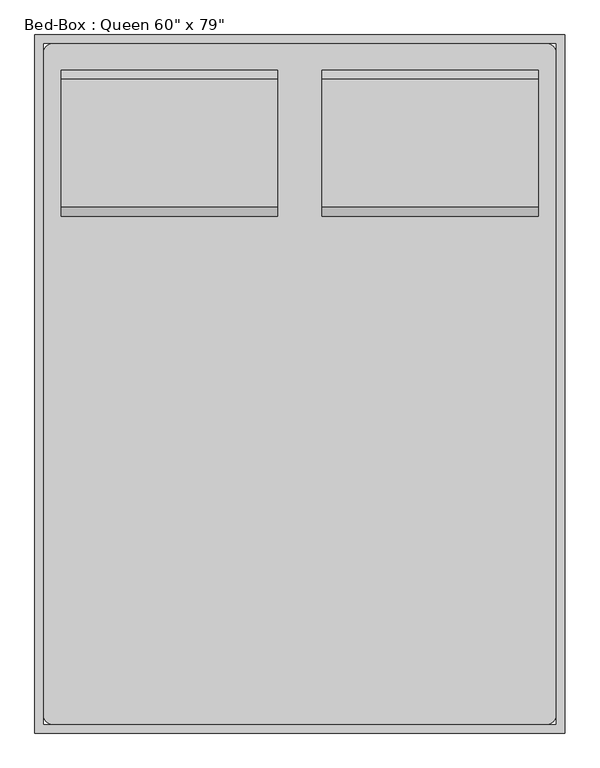
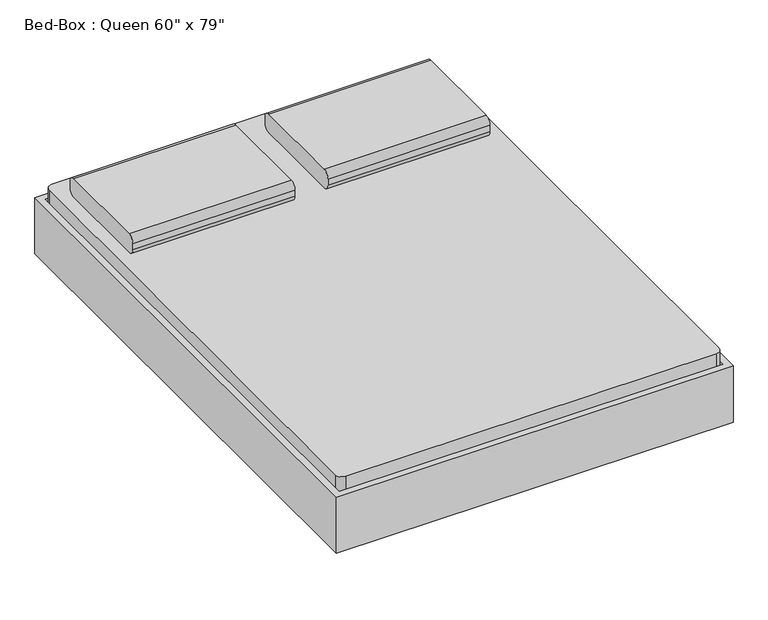
"""IFC4 building model written with IfcOpenShell, lengths in millimetres: furniture geometry."""

from ifc_helpers import new_model, si_unit, point, frame, frame_2d, origin, place, context, project, spatial, polyline, circle_curve, trimmed, segment, composite_curve, outline, extrude, source, transform, mapped, element, save
from ifc_brep_helpers import plane_surface, cylinder_surface, revolved_surface, advanced_brep


def furniture_1d2926bd(model_context):
    return source(origin(), model_context, "Body", "SolidModel", [
        extrude(outline(composite_curve([segment(polyline([(641.8704918, 406.4), (273.5704918, 406.4)]), True, "CONTINUOUS"), segment(trimmed(circle_curve(frame_2d((273.5704918, 431.8)), 25.4), [point((273.5704918, 406.4))], [point((248.1704918, 431.8))], False, "CARTESIAN"), True, "CONTINUOUS"), segment(polyline([(248.1704918, 431.8), (248.1704918, 457.2)]), True, "CONTINUOUS"), segment(trimmed(circle_curve(frame_2d((273.5704918, 457.2)), 25.4), [point((248.1704918, 457.2))], [point((273.5704918, 482.6))], False, "CARTESIAN"), True, "CONTINUOUS"), segment(polyline([(273.5704918, 482.6), (641.8704918, 482.6)]), True, "CONTINUOUS"), segment(trimmed(circle_curve(frame_2d((641.8704918, 457.2)), 25.4), [point((641.8704918, 482.6))], [point((667.2704918, 457.2))], False, "CARTESIAN"), True, "CONTINUOUS"), segment(polyline([(667.2704918, 457.2), (667.2704918, 431.8)]), True, "CONTINUOUS"), segment(trimmed(circle_curve(frame_2d((641.8704918, 431.8)), 25.4), [point((667.2704918, 431.8))], [point((641.8704918, 406.4))], False, "CARTESIAN"), True, "CONTINUOUS")], self_intersect=False)), frame((402.652459, 0.0, 0.0), z_axis=(1.0, 0.0, 0.0), x_axis=(0.0, 1.0, 0.0)), (0.0, 0.0, 1.0), 622.3),
        extrude(outline(composite_curve([segment(polyline([(641.8704918, 406.4), (273.5704918, 406.4)]), True, "CONTINUOUS"), segment(trimmed(circle_curve(frame_2d((273.5704918, 431.8)), 25.4), [point((273.5704918, 406.4))], [point((248.1704918, 431.8))], False, "CARTESIAN"), True, "CONTINUOUS"), segment(polyline([(248.1704918, 431.8), (248.1704918, 457.2)]), True, "CONTINUOUS"), segment(trimmed(circle_curve(frame_2d((273.5704918, 457.2)), 25.4), [point((248.1704918, 457.2))], [point((273.5704918, 482.6))], False, "CARTESIAN"), True, "CONTINUOUS"), segment(polyline([(273.5704918, 482.6), (641.8704918, 482.6)]), True, "CONTINUOUS"), segment(trimmed(circle_curve(frame_2d((641.8704918, 457.2)), 25.4), [point((641.8704918, 482.6))], [point((667.2704918, 457.2))], False, "CARTESIAN"), True, "CONTINUOUS"), segment(polyline([(667.2704918, 457.2), (667.2704918, 431.8)]), True, "CONTINUOUS"), segment(trimmed(circle_curve(frame_2d((641.8704918, 431.8)), 25.4), [point((667.2704918, 431.8))], [point((641.8704918, 406.4))], False, "CARTESIAN"), True, "CONTINUOUS")], self_intersect=False)), frame((-346.647541, 0.0, 0.0), z_axis=(1.0, 0.0, 0.0), x_axis=(0.0, 1.0, 0.0)), (0.0, 0.0, 1.0), 622.3),
        advanced_brep(
        [(-397.1231784, 514.8704918, 177.8), (-397.1231784, 438.6704918, 177.8), (-397.1231784, 438.6704918, 196.85), (-397.1231784, 514.8704918, 196.85), (-346.3231784, 514.8704918, 177.8), (-346.3231784, 438.6704918, 177.8), (-334.1869899, 438.6704918, 196.85), (-334.1869899, 514.8704918, 196.85), (-270.2523099, 514.8704918, 14.6654962), (-270.2523099, 438.6704918, 14.6654962), (-252.9871466, 438.6704918, 22.716374), (-252.9871466, 514.8704918, 22.716374), (-247.2320921, 438.6704918, 0.0), (-247.2320921, 514.8704918, 0.0), (-247.2320921, 438.6704918, 19.05), (-247.2320921, 514.8704918, 19.05), (-168.6195862, 514.8704918, 0.0), (-168.6195862, 438.6704918, 0.0), (-168.6195862, 438.6704918, 19.05), (-168.6195862, 514.8704918, 19.05), (-155.9195862, 438.6704918, 3.4029547), (-155.9195862, 514.8704918, 3.4029547), (-165.4445862, 438.6704918, 19.9007387), (-165.4445862, 514.8704918, 19.9007387), (-95.822541, 514.8704918, 38.1), (-95.822541, 438.6704918, 38.1), (-100.9269731, 438.6704918, 57.15), (-100.9269731, 514.8704918, 57.15), (774.4518216, 514.8704918, 38.1), (774.4518216, 438.6704918, 38.1), (779.5562537, 438.6704918, 57.15), (779.5562537, 514.8704918, 57.15), (834.5488669, 514.8704918, 3.4029547), (834.5488669, 438.6704918, 3.4029547), (844.0738669, 438.6704918, 19.9007387), (844.0738669, 514.8704918, 19.9007387), (847.2488669, 438.6704918, 0.0), (847.2488669, 514.8704918, 0.0), (847.2488669, 438.6704918, 19.05), (847.2488669, 514.8704918, 19.05), (925.8613728, 514.8704918, 0.0), (925.8613728, 438.6704918, 0.0), (925.8613728, 438.6704918, 19.05), (925.8613728, 514.8704918, 19.05), (948.8815906, 438.6704918, 14.6654962), (948.8815906, 514.8704918, 14.6654962), (931.6164272, 438.6704918, 22.716374), (931.6164272, 514.8704918, 22.716374), (1024.952459, 514.8704918, 177.8), (1024.952459, 438.6704918, 177.8), (1012.8162705, 438.6704918, 196.85), (1012.8162705, 514.8704918, 196.85), (1075.752459, 514.8704918, 177.8), (1075.752459, 514.8704918, 196.85), (1075.752459, 438.6704918, 196.85), (1075.752459, 438.6704918, 177.8)],
        [
            (0, 1),
            (1, 2),
            (2, 3),
            (3, 0),
            (0, 4),
            (4, 5),
            (5, 1),
            (5, 6),
            (6, 2),
            (6, 7),
            (7, 3),
            (7, 4),
            (4, 8),
            (8, 9),
            (9, 5),
            (9, 10),
            (10, 6),
            (10, 11),
            (11, 7),
            (11, 8),
            (12, 9, circle_curve(frame((-247.2320921, 438.6704918, 25.4), z_axis=(0.0, 1.0, 0.0), x_axis=(-0.9063077870366486, 0.0, -0.42261826174070233)), 25.4)),
            (8, 13, circle_curve(frame((-247.2320921, 514.8704918, 25.4), z_axis=(0.0, -1.0, 0.0), x_axis=(-0.9063077870366486, 0.0, -0.42261826174070233)), 25.4)),
            (13, 12),
            (14, 10, circle_curve(frame((-247.2320921, 438.6704918, 25.4), z_axis=(0.0, 1.0, 0.0), x_axis=(-0.9063077870366486, 0.0, -0.42261826174070233)), 6.35)),
            (12, 14),
            (15, 11, circle_curve(frame((-247.2320921, 514.8704918, 25.4), z_axis=(0.0, 1.0, 0.0), x_axis=(-0.9063077870366486, 0.0, -0.42261826174070233)), 6.35)),
            (14, 15),
            (15, 13),
            (13, 16),
            (16, 17),
            (17, 12),
            (17, 18),
            (18, 14),
            (18, 19),
            (19, 15),
            (19, 16),
            (20, 17, circle_curve(frame((-168.6195862, 438.6704918, 25.4), z_axis=(0.0, 1.0, 0.0), x_axis=(0.0, 0.0, -1.0)), 25.4)),
            (16, 21, circle_curve(frame((-168.6195862, 514.8704918, 25.4), z_axis=(0.0, -1.0, 0.0), x_axis=(0.0, 0.0, -1.0)), 25.4)),
            (21, 20),
            (22, 18, circle_curve(frame((-168.6195862, 438.6704918, 25.4), z_axis=(0.0, 1.0, 0.0), x_axis=(0.0, 0.0, -1.0)), 6.35)),
            (20, 22),
            (23, 19, circle_curve(frame((-168.6195862, 514.8704918, 25.4), z_axis=(0.0, 1.0, 0.0), x_axis=(0.0, 0.0, -1.0)), 6.35)),
            (22, 23),
            (23, 21),
            (21, 24),
            (24, 25),
            (25, 20),
            (25, 26),
            (26, 22),
            (26, 27),
            (27, 23),
            (27, 24),
            (24, 28),
            (28, 29),
            (29, 25),
            (29, 30),
            (30, 26),
            (30, 31),
            (31, 27),
            (31, 28),
            (28, 32),
            (32, 33),
            (33, 29),
            (33, 34),
            (34, 30),
            (34, 35),
            (35, 31),
            (35, 32),
            (36, 33, circle_curve(frame((847.2488669, 438.6704918, 25.4), z_axis=(0.0, 1.0, 0.0), x_axis=(-0.5000000000000463, 0.0, -0.8660254037844118)), 25.4)),
            (32, 37, circle_curve(frame((847.2488669, 514.8704918, 25.4), z_axis=(0.0, -1.0, 0.0), x_axis=(-0.5000000000000463, 0.0, -0.8660254037844118)), 25.4)),
            (37, 36),
            (38, 34, circle_curve(frame((847.2488669, 438.6704918, 25.4), z_axis=(0.0, 1.0, 0.0), x_axis=(-0.5000000000000463, 0.0, -0.8660254037844118)), 6.35)),
            (36, 38),
            (39, 35, circle_curve(frame((847.2488669, 514.8704918, 25.4), z_axis=(0.0, 1.0, 0.0), x_axis=(-0.5000000000000463, 0.0, -0.8660254037844118)), 6.35)),
            (38, 39),
            (39, 37),
            (37, 40),
            (40, 41),
            (41, 36),
            (41, 42),
            (42, 38),
            (42, 43),
            (43, 39),
            (43, 40),
            (44, 41, circle_curve(frame((925.8613728, 438.6704918, 25.4), z_axis=(0.0, 1.0, 0.0), x_axis=(0.0, 0.0, -1.0)), 25.4)),
            (40, 45, circle_curve(frame((925.8613728, 514.8704918, 25.4), z_axis=(0.0, -1.0, 0.0), x_axis=(0.0, 0.0, -1.0)), 25.4)),
            (45, 44),
            (46, 42, circle_curve(frame((925.8613728, 438.6704918, 25.4), z_axis=(0.0, 1.0, 0.0), x_axis=(0.0, 0.0, -1.0)), 6.35)),
            (44, 46),
            (47, 43, circle_curve(frame((925.8613728, 514.8704918, 25.4), z_axis=(0.0, 1.0, 0.0), x_axis=(0.0, 0.0, -1.0)), 6.35)),
            (46, 47),
            (47, 45),
            (45, 48),
            (48, 49),
            (49, 44),
            (49, 50),
            (50, 46),
            (50, 51),
            (51, 47),
            (51, 48),
            (52, 53),
            (53, 54),
            (54, 55),
            (55, 52),
            (48, 52),
            (55, 49),
            (54, 50),
            (53, 51),
        ],
        [
            plane_surface(frame((-397.1231784, 768.8704918, -152.9490627), z_axis=(-1.0, 0.0, 0.0), x_axis=(0.0, 1.0, 0.0))),
            plane_surface(frame((-397.1231784, 514.8704918, 177.8), z_axis=(0.0, 0.0, -1.0), x_axis=(1.0, 0.0, 0.0))),
            plane_surface(frame((-397.1231784, 438.6704918, 177.8), z_axis=(0.0, -1.0, 0.0), x_axis=(1.0, 0.0, 0.0))),
            plane_surface(frame((-397.1231784, 438.6704918, 196.85), z_axis=(0.0, 0.0, 1.0), x_axis=(1.0, 0.0, 0.0))),
            plane_surface(frame((-397.1231784, 514.8704918, 196.85), z_axis=(0.0, 1.0, 0.0), x_axis=(1.0, 0.0, 0.0))),
            plane_surface(frame((-346.3231784, 514.8704918, 177.8), z_axis=(-0.9063077870366485, 0.0, -0.4226182617407027), x_axis=(0.4226182617407027, 0.0, -0.9063077870366485))),
            plane_surface(frame((-346.3231784, 438.6704918, 177.8), z_axis=(0.0, -1.0, 0.0), x_axis=(0.4226182617407025, 0.0, -0.9063077870366486))),
            plane_surface(frame((-334.1869899, 438.6704918, 196.85), z_axis=(0.9063077870366484, 0.0, 0.4226182617407028), x_axis=(0.4226182617407028, 0.0, -0.9063077870366484))),
            plane_surface(frame((-334.1869899, 514.8704918, 196.85), z_axis=(0.0, 1.0, 0.0), x_axis=(0.42261826174070277, 0.0, -0.9063077870366485))),
            cylinder_surface(frame((-247.2320921, 768.8704918, 25.4), z_axis=(0.0, -1.0, 0.0), x_axis=(-0.9063077870366486, 0.0, -0.42261826174070233)), 25.4),
            plane_surface(frame((-247.2320921, 438.6704918, 25.4), z_axis=(0.0, -1.0, 0.0), x_axis=(-0.9063077870366486, 0.0, -0.42261826174070233))),
            revolved_surface(polyline([(-252.9871465476827, 438.6704918, 22.71637403794654), (-252.9871465476827, 514.8704918, 22.71637403794654)]), (-247.2320921, 768.8704918, 25.4), (0.0, -1.0, 0.0)),
            plane_surface(frame((-247.2320921, 514.8704918, 25.4), z_axis=(0.0, 1.0, 0.0), x_axis=(-0.9063077870366486, 0.0, -0.42261826174070233))),
            plane_surface(frame((-247.2320921, 514.8704918, 0.0), z_axis=(0.0, 0.0, -1.0), x_axis=(1.0, 0.0, 0.0))),
            plane_surface(frame((-247.2320921, 438.6704918, 0.0), z_axis=(0.0, -1.0, 0.0), x_axis=(1.0, 0.0, 0.0))),
            plane_surface(frame((-247.2320921, 438.6704918, 19.05), z_axis=(0.0, 0.0, 1.0), x_axis=(1.0, 0.0, 0.0))),
            plane_surface(frame((-247.2320921, 514.8704918, 19.05), z_axis=(0.0, 1.0, 0.0), x_axis=(1.0, 0.0, 0.0))),
            cylinder_surface(frame((-168.6195862, 768.8704918, 25.4), z_axis=(0.0, -1.0, 0.0), x_axis=(0.0, 0.0, -1.0)), 25.4),
            plane_surface(frame((-168.6195862, 438.6704918, 25.4), z_axis=(0.0, -1.0, 0.0), x_axis=(0.0, 0.0, -1.0))),
            revolved_surface(polyline([(-168.6195862, 438.6704918, 19.049999999999997), (-168.6195862, 514.8704918, 19.049999999999997)]), (-168.6195862, 768.8704918, 25.4), (0.0, -1.0, 0.0)),
            plane_surface(frame((-168.6195862, 514.8704918, 25.4), z_axis=(0.0, 1.0, 0.0), x_axis=(0.0, 0.0, -1.0))),
            plane_surface(frame((-155.9195862, 514.8704918, 3.4029547), z_axis=(0.49999999999988004, 0.0, -0.866025403784508), x_axis=(0.866025403784508, 0.0, 0.49999999999988004))),
            plane_surface(frame((-155.9195862, 438.6704918, 3.4029547), z_axis=(0.0, -1.0, 0.0), x_axis=(0.8660254037845078, 0.0, 0.49999999999988026))),
            plane_surface(frame((-165.4445862, 438.6704918, 19.9007387), z_axis=(-0.4999999999998799, 0.0, 0.866025403784508), x_axis=(0.866025403784508, 0.0, 0.4999999999998799))),
            plane_surface(frame((-165.4445862, 514.8704918, 19.9007387), z_axis=(0.0, 1.0, 0.0), x_axis=(0.8660254037845075, 0.0, 0.49999999999988076))),
            plane_surface(frame((-95.822541, 514.8704918, 38.1), z_axis=(0.0, 0.0, -1.0), x_axis=(1.0, 0.0, 0.0))),
            plane_surface(frame((-95.822541, 438.6704918, 38.1), z_axis=(0.0, -1.0, 0.0), x_axis=(1.0, 0.0, 0.0))),
            plane_surface(frame((-100.9269731, 438.6704918, 57.15), z_axis=(0.0, 0.0, 1.0), x_axis=(1.0, 0.0, 0.0))),
            plane_surface(frame((-100.9269731, 514.8704918, 57.15), z_axis=(0.0, 1.0, 0.0), x_axis=(1.0, 0.0, 0.0))),
            plane_surface(frame((774.4518216, 514.8704918, 38.1), z_axis=(-0.5000000000000455, 0.0, -0.8660254037844125), x_axis=(0.8660254037844125, 0.0, -0.5000000000000455))),
            plane_surface(frame((774.4518216, 438.6704918, 38.1), z_axis=(0.0, -1.0, 0.0), x_axis=(0.866025403784412, 0.0, -0.5000000000000463))),
            plane_surface(frame((779.5562537, 438.6704918, 57.15), z_axis=(0.5000000000000466, 0.0, 0.8660254037844117), x_axis=(0.8660254037844117, 0.0, -0.5000000000000466))),
            plane_surface(frame((779.5562537, 514.8704918, 57.15), z_axis=(0.0, 1.0, 0.0), x_axis=(0.8660254037844115, 0.0, -0.5000000000000471))),
            cylinder_surface(frame((847.2488669, 768.8704918, 25.4), z_axis=(0.0, -1.0, 0.0), x_axis=(-0.5000000000000463, 0.0, -0.8660254037844118)), 25.4),
            plane_surface(frame((847.2488669, 438.6704918, 25.4), z_axis=(0.0, -1.0000000000000002, 0.0), x_axis=(-0.5000000000000464, 0.0, -0.866025403784412))),
            revolved_surface(polyline([(844.0738668999998, 438.6704918, 19.90073868596898), (844.0738668999998, 514.8704918, 19.90073868596898)]), (847.2488669, 768.8704918, 25.4), (0.0, -1.0, 0.0)),
            plane_surface(frame((847.2488669, 514.8704918, 25.4), z_axis=(0.0, 1.0000000000000002, 0.0), x_axis=(-0.5000000000000464, 0.0, -0.866025403784412))),
            plane_surface(frame((847.2488669, 514.8704918, 0.0), z_axis=(0.0, 0.0, -1.0), x_axis=(1.0, 0.0, 0.0))),
            plane_surface(frame((847.2488669, 438.6704918, 0.0), z_axis=(0.0, -1.0, 0.0), x_axis=(1.0, 0.0, 0.0))),
            plane_surface(frame((847.2488669, 438.6704918, 19.05), z_axis=(0.0, 0.0, 1.0), x_axis=(1.0, 0.0, 0.0))),
            plane_surface(frame((847.2488669, 514.8704918, 19.05), z_axis=(0.0, 1.0, 0.0), x_axis=(1.0, 0.0, 0.0))),
            cylinder_surface(frame((925.8613728, 768.8704918, 25.4), z_axis=(0.0, -1.0, 0.0), x_axis=(0.0, 0.0, -1.0)), 25.4),
            plane_surface(frame((925.8613728, 438.6704918, 25.4), z_axis=(0.0, -1.0, 0.0), x_axis=(0.0, 0.0, -1.0))),
            revolved_surface(polyline([(925.8613728, 438.6704918, 19.049999999999997), (925.8613728, 514.8704918, 19.049999999999997)]), (925.8613728, 768.8704918, 25.4), (0.0, -1.0, 0.0)),
            plane_surface(frame((925.8613728, 514.8704918, 25.4), z_axis=(0.0, 1.0, 0.0), x_axis=(0.0, 0.0, -1.0))),
            plane_surface(frame((948.8815906, 514.8704918, 14.6654962), z_axis=(0.90630778703668, 0.0, -0.42261826174063505), x_axis=(0.42261826174063505, 0.0, 0.90630778703668))),
            plane_surface(frame((948.8815906, 438.6704918, 14.6654962), z_axis=(0.0, -1.0, 0.0), x_axis=(0.42261826174063566, 0.0, 0.9063077870366797))),
            plane_surface(frame((931.6164272, 438.6704918, 22.716374), z_axis=(-0.9063077870366801, 0.0, 0.42261826174063477), x_axis=(0.42261826174063477, 0.0, 0.9063077870366801))),
            plane_surface(frame((931.6164272, 514.8704918, 22.716374), z_axis=(0.0, 1.0, 0.0), x_axis=(0.4226182617406345, 0.0, 0.9063077870366802))),
            plane_surface(frame((1075.752459, 768.8704918, -152.9490627), z_axis=(1.0, 0.0, 0.0), x_axis=(0.0, 1.0, 0.0))),
            plane_surface(frame((1024.952459, 514.8704918, 177.8), z_axis=(0.0, 0.0, -1.0), x_axis=(1.0, 0.0, 0.0))),
            plane_surface(frame((1024.952459, 438.6704918, 177.8), z_axis=(0.0, -1.0, 0.0), x_axis=(1.0, 0.0, 0.0))),
            plane_surface(frame((1012.8162705, 438.6704918, 196.85), z_axis=(0.0, 0.0, 1.0), x_axis=(1.0, 0.0, 0.0))),
            plane_surface(frame((1012.8162705, 514.8704918, 196.85), z_axis=(0.0, 1.0, 0.0), x_axis=(1.0, 0.0, 0.0))),
        ],
        [
            (0, [[1, 2, 3, 4]]),
            (1, [[-1, 5, 6, 7]]),
            (2, [[-2, -7, 8, 9]]),
            (3, [[-3, -9, 10, 11]]),
            (4, [[-4, -11, 12, -5]]),
            (5, [[-6, 13, 14, 15]]),
            (6, [[-8, -15, 16, 17]]),
            (7, [[-10, -17, 18, 19]]),
            (8, [[-12, -19, 20, -13]]),
            (9, [[21, -14, 22, 23]]),
            (10, [[24, -16, -21, 25]]),
            (11, [[26, -18, -24, 27]]),
            (12, [[-22, -20, -26, 28]]),
            (13, [[-23, 29, 30, 31]]),
            (14, [[-25, -31, 32, 33]]),
            (15, [[-27, -33, 34, 35]]),
            (16, [[-28, -35, 36, -29]]),
            (17, [[37, -30, 38, 39]]),
            (18, [[40, -32, -37, 41]]),
            (19, [[42, -34, -40, 43]]),
            (20, [[-38, -36, -42, 44]]),
            (21, [[-39, 45, 46, 47]]),
            (22, [[-41, -47, 48, 49]]),
            (23, [[-43, -49, 50, 51]]),
            (24, [[-44, -51, 52, -45]]),
            (25, [[-46, 53, 54, 55]]),
            (26, [[-48, -55, 56, 57]]),
            (27, [[-50, -57, 58, 59]]),
            (28, [[-52, -59, 60, -53]]),
            (29, [[-54, 61, 62, 63]]),
            (30, [[-56, -63, 64, 65]]),
            (31, [[-58, -65, 66, 67]]),
            (32, [[-60, -67, 68, -61]]),
            (33, [[69, -62, 70, 71]]),
            (34, [[72, -64, -69, 73]]),
            (35, [[74, -66, -72, 75]]),
            (36, [[-70, -68, -74, 76]]),
            (37, [[-71, 77, 78, 79]]),
            (38, [[-73, -79, 80, 81]]),
            (39, [[-75, -81, 82, 83]]),
            (40, [[-76, -83, 84, -77]]),
            (41, [[85, -78, 86, 87]]),
            (42, [[88, -80, -85, 89]]),
            (43, [[90, -82, -88, 91]]),
            (44, [[-86, -84, -90, 92]]),
            (45, [[-87, 93, 94, 95]]),
            (46, [[-89, -95, 96, 97]]),
            (47, [[-91, -97, 98, 99]]),
            (48, [[-92, -99, 100, -93]]),
            (49, [[101, 102, 103, 104]]),
            (50, [[-94, 105, -104, 106]]),
            (51, [[-96, -106, -103, 107]]),
            (52, [[-98, -107, -102, 108]]),
            (53, [[-100, -108, -101, -105]]),
        ],
    ),
        extrude(outline(composite_curve([segment(polyline([(-372.047541, 743.4704918), (1050.352459, 743.4704918)]), True, "CONTINUOUS"), segment(trimmed(circle_curve(frame_2d((1050.352459, 718.0704918)), 25.4), [point((1050.352459, 743.4704918))], [point((1075.752459, 718.0704918))], False, "CARTESIAN"), True, "CONTINUOUS"), segment(polyline([(1075.752459, 718.0704918), (1075.752459, -1186.9295082)]), True, "CONTINUOUS"), segment(trimmed(circle_curve(frame_2d((1050.352459, -1186.9295082)), 25.4), [point((1075.752459, -1186.9295082))], [point((1050.352459, -1212.3295082))], False, "CARTESIAN"), True, "CONTINUOUS"), segment(polyline([(1050.352459, -1212.3295082), (-372.047541, -1212.3295082)]), True, "CONTINUOUS"), segment(trimmed(circle_curve(frame_2d((-372.047541, -1186.9295082)), 25.4), [point((-372.047541, -1212.3295082))], [point((-397.447541, -1186.9295082))], False, "CARTESIAN"), True, "CONTINUOUS"), segment(polyline([(-397.447541, -1186.9295082), (-397.447541, 718.0704918)]), True, "CONTINUOUS"), segment(trimmed(circle_curve(frame_2d((-372.047541, 718.0704918)), 25.4), [point((-397.447541, 718.0704918))], [point((-372.047541, 743.4704918))], False, "CARTESIAN"), True, "CONTINUOUS")], self_intersect=False)), frame((0.0, 0.0, 203.2), z_axis=(0.0, 0.0, 1.0), x_axis=(1.0, 0.0, 0.0)), (0.0, 0.0, 1.0), 203.2),
        advanced_brep(
        [(-397.447541, -932.9295082, 196.85), (-397.447541, -932.9295082, 177.8), (-397.447541, -1009.1295082, 177.8), (-397.447541, -1009.1295082, 196.85), (-334.5113525, -932.9295082, 196.85), (-346.647541, -932.9295082, 177.8), (-346.647541, -1009.1295082, 177.8), (-334.5113525, -1009.1295082, 196.85), (-253.3115092, -932.9295082, 22.716374), (-270.5766725, -932.9295082, 14.6654962), (-270.5766725, -1009.1295082, 14.6654962), (-253.3115092, -1009.1295082, 22.716374), (-247.5564547, -932.9295082, 0.0), (-247.5564547, -932.9295082, 19.05), (-247.5564547, -1009.1295082, 0.0), (-247.5564547, -1009.1295082, 19.05), (-168.9439489, -932.9295082, 19.05), (-168.9439489, -932.9295082, 0.0), (-168.9439489, -1009.1295082, 0.0), (-168.9439489, -1009.1295082, 19.05), (-156.2439489, -932.9295082, 3.4029547), (-165.7689489, -932.9295082, 19.9007387), (-156.2439489, -1009.1295082, 3.4029547), (-165.7689489, -1009.1295082, 19.9007387), (-101.2513357, -932.9295082, 57.15), (-96.1469036, -932.9295082, 38.1), (-96.1469036, -1009.1295082, 38.1), (-101.2513357, -1009.1295082, 57.15), (779.5562537, -932.9295082, 57.15), (774.4518216, -932.9295082, 38.1), (774.4518216, -1009.1295082, 38.1), (779.5562537, -1009.1295082, 57.15), (844.0738669, -932.9295082, 19.9007387), (834.5488669, -932.9295082, 3.4029547), (834.5488669, -1009.1295082, 3.4029547), (844.0738669, -1009.1295082, 19.9007387), (847.2488669, -932.9295082, 0.0), (847.2488669, -932.9295082, 19.05), (847.2488669, -1009.1295082, 0.0), (847.2488669, -1009.1295082, 19.05), (925.8613728, -932.9295082, 19.05), (925.8613728, -932.9295082, 0.0), (925.8613728, -1009.1295082, 0.0), (925.8613728, -1009.1295082, 19.05), (948.8815906, -932.9295082, 14.6654962), (931.6164272, -932.9295082, 22.716374), (948.8815906, -1009.1295082, 14.6654962), (931.6164272, -1009.1295082, 22.716374), (1012.8162705, -932.9295082, 196.85), (1024.952459, -932.9295082, 177.8), (1024.952459, -1009.1295082, 177.8), (1012.8162705, -1009.1295082, 196.85), (1075.752459, -932.9295082, 196.85), (1075.752459, -1009.1295082, 196.85), (1075.752459, -1009.1295082, 177.8), (1075.752459, -932.9295082, 177.8)],
        [
            (0, 1),
            (1, 2),
            (2, 3),
            (3, 0),
            (0, 4),
            (4, 5),
            (5, 1),
            (5, 6),
            (6, 2),
            (6, 7),
            (7, 3),
            (7, 4),
            (4, 8),
            (8, 9),
            (9, 5),
            (9, 10),
            (10, 6),
            (10, 11),
            (11, 7),
            (11, 8),
            (12, 9, circle_curve(frame((-247.5564547, -932.9295082, 25.4), z_axis=(0.0, 1.0, 0.0), x_axis=(-0.906307787036663, 0.0, -0.4226182617406713)), 25.4)),
            (8, 13, circle_curve(frame((-247.5564547, -932.9295082, 25.4), z_axis=(0.0, -1.0, 0.0), x_axis=(-0.906307787036663, 0.0, -0.4226182617406713)), 6.35)),
            (13, 12),
            (14, 10, circle_curve(frame((-247.5564547, -1009.1295082, 25.4), z_axis=(0.0, 1.0, 0.0), x_axis=(-0.906307787036663, 0.0, -0.4226182617406713)), 25.4)),
            (12, 14),
            (15, 11, circle_curve(frame((-247.5564547, -1009.1295082, 25.4), z_axis=(0.0, 1.0, 0.0), x_axis=(-0.906307787036663, 0.0, -0.4226182617406713)), 6.35)),
            (14, 15),
            (15, 13),
            (13, 16),
            (16, 17),
            (17, 12),
            (17, 18),
            (18, 14),
            (18, 19),
            (19, 15),
            (19, 16),
            (20, 17, circle_curve(frame((-168.9439489, -932.9295082, 25.4), z_axis=(0.0, 1.0, 0.0), x_axis=(0.0, 0.0, -1.0)), 25.4)),
            (16, 21, circle_curve(frame((-168.9439489, -932.9295082, 25.4), z_axis=(0.0, -1.0, 0.0), x_axis=(0.0, 0.0, -1.0)), 6.35)),
            (21, 20),
            (22, 18, circle_curve(frame((-168.9439489, -1009.1295082, 25.4), z_axis=(0.0, 1.0, 0.0), x_axis=(0.0, 0.0, -1.0)), 25.4)),
            (20, 22),
            (23, 19, circle_curve(frame((-168.9439489, -1009.1295082, 25.4), z_axis=(0.0, 1.0, 0.0), x_axis=(0.0, 0.0, -1.0)), 6.35)),
            (22, 23),
            (23, 21),
            (21, 24),
            (24, 25),
            (25, 20),
            (25, 26),
            (26, 22),
            (26, 27),
            (27, 23),
            (27, 24),
            (24, 28),
            (28, 29),
            (29, 25),
            (29, 30),
            (30, 26),
            (30, 31),
            (31, 27),
            (31, 28),
            (28, 32),
            (32, 33),
            (33, 29),
            (33, 34),
            (34, 30),
            (34, 35),
            (35, 31),
            (35, 32),
            (36, 33, circle_curve(frame((847.2488669, -932.9295082, 25.4), z_axis=(0.0, 1.0, 0.0), x_axis=(-0.5000000000000479, 0.0, -0.866025403784411)), 25.4)),
            (32, 37, circle_curve(frame((847.2488669, -932.9295082, 25.4), z_axis=(0.0, -1.0, 0.0), x_axis=(-0.5000000000000479, 0.0, -0.866025403784411)), 6.35)),
            (37, 36),
            (38, 34, circle_curve(frame((847.2488669, -1009.1295082, 25.4), z_axis=(0.0, 1.0, 0.0), x_axis=(-0.5000000000000479, 0.0, -0.866025403784411)), 25.4)),
            (36, 38),
            (39, 35, circle_curve(frame((847.2488669, -1009.1295082, 25.4), z_axis=(0.0, 1.0, 0.0), x_axis=(-0.5000000000000479, 0.0, -0.866025403784411)), 6.35)),
            (38, 39),
            (39, 37),
            (37, 40),
            (40, 41),
            (41, 36),
            (41, 42),
            (42, 38),
            (42, 43),
            (43, 39),
            (43, 40),
            (44, 41, circle_curve(frame((925.8613728, -932.9295082, 25.4), z_axis=(0.0, 1.0, 0.0), x_axis=(0.0, 0.0, -1.0)), 25.4)),
            (40, 45, circle_curve(frame((925.8613728, -932.9295082, 25.4), z_axis=(0.0, -1.0, 0.0), x_axis=(0.0, 0.0, -1.0)), 6.35)),
            (45, 44),
            (46, 42, circle_curve(frame((925.8613728, -1009.1295082, 25.4), z_axis=(0.0, 1.0, 0.0), x_axis=(0.0, 0.0, -1.0)), 25.4)),
            (44, 46),
            (47, 43, circle_curve(frame((925.8613728, -1009.1295082, 25.4), z_axis=(0.0, 1.0, 0.0), x_axis=(0.0, 0.0, -1.0)), 6.35)),
            (46, 47),
            (47, 45),
            (45, 48),
            (48, 49),
            (49, 44),
            (49, 50),
            (50, 46),
            (50, 51),
            (51, 47),
            (51, 48),
            (52, 53),
            (53, 54),
            (54, 55),
            (55, 52),
            (48, 52),
            (55, 49),
            (54, 50),
            (53, 51),
        ],
        [
            plane_surface(frame((-397.447541, -1237.7295082, -127.5947323), z_axis=(-1.0, 0.0, 0.0), x_axis=(0.0, 1.0, 0.0))),
            plane_surface(frame((-397.447541, -932.9295082, 196.85), z_axis=(0.0, 1.0, 0.0), x_axis=(1.0, 0.0, 0.0))),
            plane_surface(frame((-397.447541, -932.9295082, 177.8), z_axis=(0.0, 0.0, -1.0), x_axis=(1.0, 0.0, 0.0))),
            plane_surface(frame((-397.447541, -1009.1295082, 177.8), z_axis=(0.0, -1.0, 0.0), x_axis=(1.0, 0.0, 0.0))),
            plane_surface(frame((-397.447541, -1009.1295082, 196.85), z_axis=(0.0, 0.0, 1.0), x_axis=(1.0, 0.0, 0.0))),
            plane_surface(frame((-334.5113525, -932.9295082, 196.85), z_axis=(0.0, 1.0, 0.0), x_axis=(0.4226182617406707, 0.0, -0.9063077870366634))),
            plane_surface(frame((-346.647541, -932.9295082, 177.8), z_axis=(-0.9063077870366635, 0.0, -0.4226182617406707), x_axis=(0.4226182617406707, 0.0, -0.9063077870366635))),
            plane_surface(frame((-346.647541, -1009.1295082, 177.8), z_axis=(0.0, -1.0, 0.0), x_axis=(0.422618261740671, 0.0, -0.9063077870366633))),
            plane_surface(frame((-334.5113525, -1009.1295082, 196.85), z_axis=(0.9063077870366633, 0.0, 0.42261826174067113), x_axis=(0.42261826174067113, 0.0, -0.9063077870366633))),
            plane_surface(frame((-247.5564547, -932.9295082, 25.4), z_axis=(0.0, 1.0, 0.0), x_axis=(-0.906307787036663, 0.0, -0.4226182617406713))),
            cylinder_surface(frame((-247.5564547, -1237.7295082, 25.4), z_axis=(0.0, -1.0, 0.0), x_axis=(-0.906307787036663, 0.0, -0.4226182617406713)), 25.4),
            plane_surface(frame((-247.5564547, -1009.1295082, 25.4), z_axis=(0.0, -1.0, 0.0), x_axis=(-0.906307787036663, 0.0, -0.4226182617406713))),
            revolved_surface(polyline([(-253.3115091476828, -1009.1295082, 22.716374037946736), (-253.3115091476828, -932.9295082, 22.716374037946736)]), (-247.5564547, -1237.7295082, 25.4), (0.0, -1.0, 0.0)),
            plane_surface(frame((-247.5564547, -932.9295082, 19.05), z_axis=(0.0, 1.0, 0.0), x_axis=(1.0, 0.0, 0.0))),
            plane_surface(frame((-247.5564547, -932.9295082, 0.0), z_axis=(0.0, 0.0, -1.0), x_axis=(1.0, 0.0, 0.0))),
            plane_surface(frame((-247.5564547, -1009.1295082, 0.0), z_axis=(0.0, -1.0, 0.0), x_axis=(1.0, 0.0, 0.0))),
            plane_surface(frame((-247.5564547, -1009.1295082, 19.05), z_axis=(0.0, 0.0, 1.0), x_axis=(1.0, 0.0, 0.0))),
            plane_surface(frame((-168.9439489, -932.9295082, 25.4), z_axis=(0.0, 1.0, 0.0), x_axis=(0.0, 0.0, -1.0))),
            cylinder_surface(frame((-168.9439489, -1237.7295082, 25.4), z_axis=(0.0, -1.0, 0.0), x_axis=(0.0, 0.0, -1.0)), 25.4),
            plane_surface(frame((-168.9439489, -1009.1295082, 25.4), z_axis=(0.0, -1.0, 0.0), x_axis=(0.0, 0.0, -1.0))),
            revolved_surface(polyline([(-168.9439489, -1009.1295082, 19.049999999999997), (-168.9439489, -932.9295082, 19.049999999999997)]), (-168.9439489, -1237.7295082, 25.4), (0.0, -1.0, 0.0)),
            plane_surface(frame((-165.7689489, -932.9295082, 19.9007387), z_axis=(0.0, 1.0, 0.0), x_axis=(0.8660254037844788, 0.0, 0.4999999999999306))),
            plane_surface(frame((-156.2439489, -932.9295082, 3.4029547), z_axis=(0.49999999999993017, 0.0, -0.866025403784479), x_axis=(0.866025403784479, 0.0, 0.49999999999993017))),
            plane_surface(frame((-156.2439489, -1009.1295082, 3.4029547), z_axis=(0.0, -1.0, 0.0), x_axis=(0.8660254037844785, 0.0, 0.49999999999993106))),
            plane_surface(frame((-165.7689489, -1009.1295082, 19.9007387), z_axis=(-0.4999999999999309, 0.0, 0.8660254037844786), x_axis=(0.8660254037844786, 0.0, 0.4999999999999309))),
            plane_surface(frame((-101.2513357, -932.9295082, 57.15), z_axis=(0.0, 1.0, 0.0), x_axis=(1.0, 0.0, 0.0))),
            plane_surface(frame((-96.1469036, -932.9295082, 38.1), z_axis=(0.0, 0.0, -1.0), x_axis=(1.0, 0.0, 0.0))),
            plane_surface(frame((-96.1469036, -1009.1295082, 38.1), z_axis=(0.0, -1.0, 0.0), x_axis=(1.0, 0.0, 0.0))),
            plane_surface(frame((-101.2513357, -1009.1295082, 57.15), z_axis=(0.0, 0.0, 1.0), x_axis=(1.0, 0.0, 0.0))),
            plane_surface(frame((779.5562537, -932.9295082, 57.15), z_axis=(0.0, 1.0000000000000002, 0.0), x_axis=(0.8660254037844106, 0.0, -0.5000000000000487))),
            plane_surface(frame((774.4518216, -932.9295082, 38.1), z_axis=(-0.5000000000000477, 0.0, -0.8660254037844112), x_axis=(0.8660254037844112, 0.0, -0.5000000000000477))),
            plane_surface(frame((774.4518216, -1009.1295082, 38.1), z_axis=(0.0, -1.0000000000000002, 0.0), x_axis=(0.8660254037844105, 0.0, -0.500000000000049))),
            plane_surface(frame((779.5562537, -1009.1295082, 57.15), z_axis=(0.5000000000000498, 0.0, 0.8660254037844098), x_axis=(0.8660254037844098, 0.0, -0.5000000000000498))),
            plane_surface(frame((847.2488669, -932.9295082, 25.4), z_axis=(0.0, 1.0000000000000002, 0.0), x_axis=(-0.500000000000048, 0.0, -0.8660254037844111))),
            cylinder_surface(frame((847.2488669, -1237.7295082, 25.4), z_axis=(0.0, -1.0, 0.0), x_axis=(-0.5000000000000479, 0.0, -0.866025403784411)), 25.4),
            plane_surface(frame((847.2488669, -1009.1295082, 25.4), z_axis=(0.0, -1.0000000000000002, 0.0), x_axis=(-0.500000000000048, 0.0, -0.8660254037844111))),
            revolved_surface(polyline([(844.0738668999998, -1009.1295082, 19.90073868596899), (844.0738668999998, -932.9295082, 19.90073868596899)]), (847.2488669, -1237.7295082, 25.4), (0.0, -1.0, 0.0)),
            plane_surface(frame((847.2488669, -932.9295082, 19.05), z_axis=(0.0, 1.0, 0.0), x_axis=(1.0, 0.0, 0.0))),
            plane_surface(frame((847.2488669, -932.9295082, 0.0), z_axis=(0.0, 0.0, -1.0), x_axis=(1.0, 0.0, 0.0))),
            plane_surface(frame((847.2488669, -1009.1295082, 0.0), z_axis=(0.0, -1.0, 0.0), x_axis=(1.0, 0.0, 0.0))),
            plane_surface(frame((847.2488669, -1009.1295082, 19.05), z_axis=(0.0, 0.0, 1.0), x_axis=(1.0, 0.0, 0.0))),
            plane_surface(frame((925.8613728, -932.9295082, 25.4), z_axis=(0.0, 1.0, 0.0), x_axis=(0.0, 0.0, -1.0))),
            cylinder_surface(frame((925.8613728, -1237.7295082, 25.4), z_axis=(0.0, -1.0, 0.0), x_axis=(0.0, 0.0, -1.0)), 25.4),
            plane_surface(frame((925.8613728, -1009.1295082, 25.4), z_axis=(0.0, -1.0, 0.0), x_axis=(0.0, 0.0, -1.0))),
            revolved_surface(polyline([(925.8613728, -1009.1295082, 19.049999999999997), (925.8613728, -932.9295082, 19.049999999999997)]), (925.8613728, -1237.7295082, 25.4), (0.0, -1.0, 0.0)),
            plane_surface(frame((931.6164272, -932.9295082, 22.716374), z_axis=(0.0, 1.0, 0.0), x_axis=(0.4226182617405411, 0.0, 0.9063077870367238))),
            plane_surface(frame((948.8815906, -932.9295082, 14.6654962), z_axis=(0.9063077870367237, 0.0, -0.4226182617405414), x_axis=(0.4226182617405414, 0.0, 0.9063077870367237))),
            plane_surface(frame((948.8815906, -1009.1295082, 14.6654962), z_axis=(0.0, -1.0, 0.0), x_axis=(0.42261826174054123, 0.0, 0.9063077870367238))),
            plane_surface(frame((931.6164272, -1009.1295082, 22.716374), z_axis=(-0.9063077870367237, 0.0, 0.4226182617405414), x_axis=(0.4226182617405414, 0.0, 0.9063077870367237))),
            plane_surface(frame((1075.752459, -1237.7295082, -127.5947323), z_axis=(1.0, 0.0, 0.0), x_axis=(0.0, 1.0, 0.0))),
            plane_surface(frame((1012.8162705, -932.9295082, 196.85), z_axis=(0.0, 1.0, 0.0), x_axis=(1.0, 0.0, 0.0))),
            plane_surface(frame((1024.952459, -932.9295082, 177.8), z_axis=(0.0, 0.0, -1.0), x_axis=(1.0, 0.0, 0.0))),
            plane_surface(frame((1024.952459, -1009.1295082, 177.8), z_axis=(0.0, -1.0, 0.0), x_axis=(1.0, 0.0, 0.0))),
            plane_surface(frame((1012.8162705, -1009.1295082, 196.85), z_axis=(0.0, 0.0, 1.0), x_axis=(1.0, 0.0, 0.0))),
        ],
        [
            (0, [[1, 2, 3, 4]]),
            (1, [[-1, 5, 6, 7]]),
            (2, [[-2, -7, 8, 9]]),
            (3, [[-3, -9, 10, 11]]),
            (4, [[-4, -11, 12, -5]]),
            (5, [[-6, 13, 14, 15]]),
            (6, [[-8, -15, 16, 17]]),
            (7, [[-10, -17, 18, 19]]),
            (8, [[-12, -19, 20, -13]]),
            (9, [[21, -14, 22, 23]]),
            (10, [[24, -16, -21, 25]]),
            (11, [[26, -18, -24, 27]]),
            (12, [[-22, -20, -26, 28]]),
            (13, [[-23, 29, 30, 31]]),
            (14, [[-25, -31, 32, 33]]),
            (15, [[-27, -33, 34, 35]]),
            (16, [[-28, -35, 36, -29]]),
            (17, [[37, -30, 38, 39]]),
            (18, [[40, -32, -37, 41]]),
            (19, [[42, -34, -40, 43]]),
            (20, [[-38, -36, -42, 44]]),
            (21, [[-39, 45, 46, 47]]),
            (22, [[-41, -47, 48, 49]]),
            (23, [[-43, -49, 50, 51]]),
            (24, [[-44, -51, 52, -45]]),
            (25, [[-46, 53, 54, 55]]),
            (26, [[-48, -55, 56, 57]]),
            (27, [[-50, -57, 58, 59]]),
            (28, [[-52, -59, 60, -53]]),
            (29, [[-54, 61, 62, 63]]),
            (30, [[-56, -63, 64, 65]]),
            (31, [[-58, -65, 66, 67]]),
            (32, [[-60, -67, 68, -61]]),
            (33, [[69, -62, 70, 71]]),
            (34, [[72, -64, -69, 73]]),
            (35, [[74, -66, -72, 75]]),
            (36, [[-70, -68, -74, 76]]),
            (37, [[-71, 77, 78, 79]]),
            (38, [[-73, -79, 80, 81]]),
            (39, [[-75, -81, 82, 83]]),
            (40, [[-76, -83, 84, -77]]),
            (41, [[85, -78, 86, 87]]),
            (42, [[88, -80, -85, 89]]),
            (43, [[90, -82, -88, 91]]),
            (44, [[-86, -84, -90, 92]]),
            (45, [[-87, 93, 94, 95]]),
            (46, [[-89, -95, 96, 97]]),
            (47, [[-91, -97, 98, 99]]),
            (48, [[-92, -99, 100, -93]]),
            (49, [[101, 102, 103, 104]]),
            (50, [[-94, 105, -104, 106]]),
            (51, [[-96, -106, -103, 107]]),
            (52, [[-98, -107, -102, 108]]),
            (53, [[-100, -108, -101, -105]]),
        ],
    ),
        extrude(outline(polyline([(1101.152459, 768.8704918), (1101.152459, -1237.7295082), (-422.847541, -1237.7295082), (-422.847541, 768.8704918), (1101.152459, 768.8704918)]), holes=[polyline([(1075.752459, 743.4704918), (-397.447541, 743.4704918), (-397.447541, -1212.3295082), (1075.752459, -1212.3295082), (1075.752459, 743.4704918)])]), frame((0.0, 0.0, 127.0), z_axis=(0.0, 0.0, 1.0), x_axis=(1.0, 0.0, 0.0)), (0.0, 0.0, 1.0), 228.6),
    ])


if __name__ == "__main__":
    model = new_model("IFC4")
    model_context = context("Model", 3, world=origin())
    ifc_project = project(units=[si_unit("LENGTHUNIT", "METRE", prefix="MILLI")], contexts=[model_context])
    site = spatial("IfcSite", under=ifc_project)
    building = spatial("IfcBuilding", under=site)
    placement = place(None, origin())
    furniture_shape = furniture_1d2926bd(model_context)
    element("IfcFurniture", 1, ObjectType="Bed-Box : Queen 60\" x 79\"", at=placement, inside=building, context=model_context, shape_type="MappedRepresentation", body=[
        mapped(furniture_shape, transform((0.0, 0.0, 0.0), x_axis=(1.0, 0.0, 0.0), y_axis=(0.0, 1.0, 0.0), z_axis=(0.0, 0.0, 1.0))),
    ])
    save(model, "model.ifc")

# Revit data of these elements
# Type "Bed-Box : Queen 60\" x 79\""
#   Assembly Code = "E2020200"
#   Length = 6' - 7"
#   Width = 5' - 0"
#   Frame Material = Birch
#   Mattress Material = Softwood, Lumber
#   Default Elevation = 0
# Element 1 (IfcFurniture, "Bed-Box : Queen 60\" x 79\"")
#   Materials on its faces: "Birch", "Softwood, Lumber"
# Materials
#   "Birch": class "Wood", colour RGB 224 178 126, transparency 0, Description = "Betula Alleghaniensis", Cost = 0
#   "Softwood, Lumber": class "Wood", colour RGB 223 192 134, transparency 0, Description = "Pinus Echinata", Cost = 0
